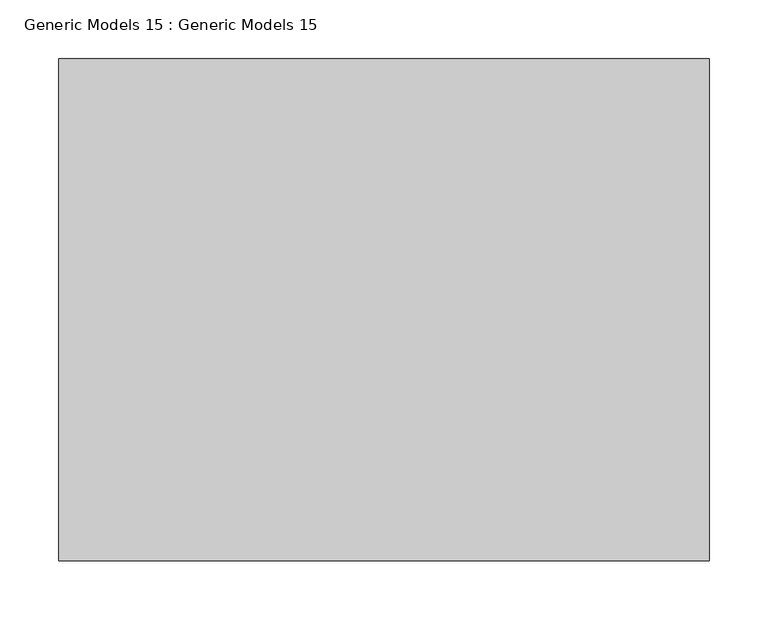
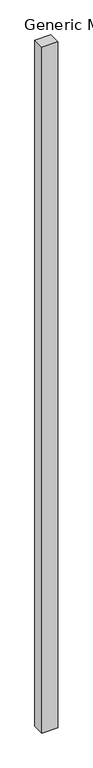
"""IFC4 building model written with IfcOpenShell, lengths in millimetres: proxy geometry, Generic Models 15 : Generic Models 15."""

from ifc_helpers import new_model, si_unit, frame, origin, place, context, project, spatial, polyline, outline, extrude, source, transform, mapped, element, save


def generic_models_15_generic_models_15_a9d5df0f(model_context):
    return source(origin(), model_context, "Body", "SweptSolid", [
        extrude(outline(polyline([(3308.0370151, -3979.0965687), (3308.0370151, -4404.8405988), (2756.2686483, -4404.8405988), (2756.2686483, -3979.0965687), (3308.0370151, -3979.0965687)])), frame((0.0, 0.0, 3411.9703205), z_axis=(0.0, 0.0, 1.0), x_axis=(1.0, 0.0, 0.0)), (0.0, 0.0, 1.0), 25149.4002945),
    ])


if __name__ == "__main__":
    model = new_model("IFC4")
    model_context = context("Model", 3, world=origin())
    ifc_project = project(units=[si_unit("LENGTHUNIT", "METRE", prefix="MILLI")], contexts=[model_context])
    site = spatial("IfcSite", under=ifc_project)
    building = spatial("IfcBuilding", under=site)
    placement = place(None, origin())
    generic_models_15_generic_models_15_shape = generic_models_15_generic_models_15_a9d5df0f(model_context)
    element("IfcBuildingElementProxy", 1, Name="Generic Models 15 : Generic Models 15", ObjectType="Generic Models 15 : Generic Models 15", at=placement, inside=building, context=model_context, shape_type="MappedRepresentation", body=[
        mapped(generic_models_15_generic_models_15_shape, transform((0.0, 0.0, 0.0), x_axis=(1.0, 0.0, 0.0), y_axis=(0.0, 1.0, 0.0), z_axis=(0.0, 0.0, 1.0))),
    ])
    save(model, "model.ifc")
